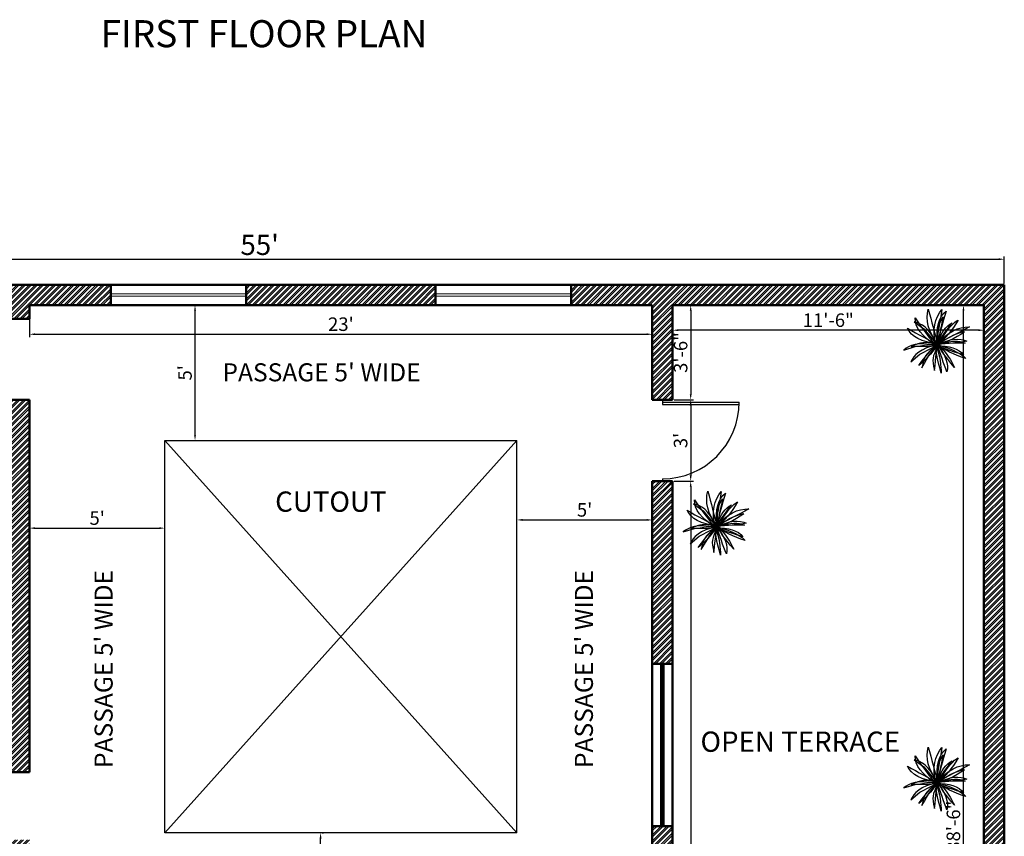
# Model space of a CAD drawing. Units: inches. Extents: x 3590 to 5167, y 65 to 1917.
# Tile 12 of 100: x 4644 to 5080, y 345 to 707. Entities that reach past the tile are written whole.
import ezdxf

# ---------------------------------------------------------------- set-up
doc = ezdxf.new("R2010")
doc.units = ezdxf.units.IN
for name, color, linetype, lineweight in [('A-ANNO-DIMS', 2, 'Continuous', 18), ('A-ANNO-TEXT', 7, 'Continuous', 25), ('A-AREA-IDEN', 7, 'Continuous', 18), ('A-DOOR', 3, 'Continuous', 25), ('A-FLOR-OTLN', 7, 'Continuous', 25), ('A-GLAZ', 4, 'Continuous', 18), ('A-WALL', 7, 'Continuous', 50), ('A-WALL-PATT', 251, 'Continuous', 13), ('L-PLNT', 94, 'Continuous', 18)]:
    doc.layers.add(name, color=color, linetype=linetype, lineweight=lineweight)
doc.layers.add('DIENHOA', color=3, linetype='Continuous')
doc.styles.get("Standard").update_dxf_attribs({"font": 'arial.ttf'})
doc.dimstyles.new('ISO-25', dxfattribs={"dimtxt": 9, "dimasz": 2.5, "dimexe": 1.25, "dimexo": 0.625, "dimtad": 1, "dimdec": 1, "dimlunit": 3, "dimtxsty": 'Standard', "dimcen": 2.5, "dimadec": 0, "dimazin": 0, "dimtfac": 1, "dimtdec": 1, "dimtmove": 0, "dimatfit": 3, "dimfxl": 1, "dimarcsym": 0})

# ---------------------------------------------------------------- blocks, each defined once
blk = doc.blocks.new('*D279')
at = {"layer": 'A-ANNO-DIMS', "color": 0, "lineweight": -2, "transparency": 16777216}
for p, q in [((4420.27, 589.68), (4420.27, 601.68)), ((4422.77, 600.43), (5077.77, 600.43)), ((5080.27, 589.68), (5080.27, 601.68))]:
    blk.add_line(p, q, dxfattribs=at)
at = {"layer": 'A-ANNO-DIMS', "color": 0, "transparency": 16777216}
for points in [[(4422.77, 600.84), (4422.77, 600.01), (4420.27, 600.43)], [(5077.77, 600.84), (5077.77, 600.01), (5080.27, 600.43)]]:
    blk.add_solid(points, dxfattribs=at)
at = {"layer": 'Defpoints', "color": 0, "transparency": 16777216}
for p in [(5080.27, 600.43), (4420.27, 589.06), (5080.27, 589.06)]:
    blk.add_point(p, dxfattribs=at)
at = {"layer": 'A-ANNO-DIMS', "color": 0, "transparency": 16777216, "insert": (4750.27, 605.63), "char_height": 9, "attachment_point": 5}
blk.add_mtext("55'", dxfattribs=at)
blk = doc.blocks.new('Cay03_mb')
at = {"layer": 'DIENHOA'}
for p, q in [((79, 504), (119, 555)), ((119, 555), (166, 599)), ((166, 599), (142, 519)), ((-365, 390), (-414, 403)), ((-414, 403), (-240, 278)), ((-315, 371), (-365, 390)), ((-264, 343), (-315, 371)), ((10, 295), (25, 374)), ((25, 374), (49, 444)), ((49, 444), (79, 504)), ((97, 366), (76, 291)), ((119, 442), (97, 366)), ((142, 519), (119, 442)), ((-211, 305), (-264, 343)), ((-240, 278), (-88, 95)), ((-158, 252), (-211, 305)), ((-104, 184), (-158, 252)), ((-50, 98), (-104, 184)), ((0, 105), (2, 206)), ((2, 206), (10, 295)), ((56, 216), (37, 142)), ((76, 291), (56, 216)), ((147, 144), (219, 200)), ((219, 200), (291, 243)), ((364, 193), (290, 155)), ((291, 243), (363, 275)), ((363, 275), (437, 297)), ((438, 231), (364, 193)), ((437, 297), (511, 310)), ((512, 271), (438, 231)), ((511, 310), (586, 314)), ((586, 314), (512, 271)), ((-345, 5), (-400, -17)), ((-299, 20), (-345, 5)), ((-255, 27), (-299, 20)), ((-208, 28), (-255, 27)), ((-153, 22), (-208, 28)), ((-83, 10), (-153, 22)), ((-88, 95), (5, -8)), ((5, -8), (-83, 10)), ((5, -8), (-50, 98)), ((5, -8), (0, 105)), ((5, -8), (76, 75)), ((20, 68), (5, -8)), ((75, 36), (5, -8)), ((5, -8), (100, 18)), ((46, 1), (5, -8)), ((37, 142), (20, 68)), ((97, 7), (46, 1)), ((145, 77), (75, 36)), ((76, 75), (147, 144)), ((155, 12), (97, 7)), ((100, 18), (182, 37)), ((217, 117), (145, 77)), ((220, 15), (155, 12)), ((182, 37), (253, 49)), ((290, 155), (217, 117)), ((289, 17), (220, 15)), ((253, 49), (315, 54)), ((362, 19), (289, 17)), ((315, 54), (369, 53)), ((436, 19), (362, 19)), ((369, 53), (419, 47)), ((419, 47), (465, 35)), ((510, 19), (436, 19)), ((465, 35), (510, 19)), ((-400, -17), (-468, -48)), ((-468, -48), (-376, -38)), ((-376, -38), (-295, -28)), ((-295, -28), (-226, -19)), ((-226, -19), (-166, -11)), ((-216, -236), (-166, -174)), ((-166, -11), (-114, -6)), ((-166, -174), (-120, -122)), ((-120, -122), (-80, -80)), ((-75, -127), (-118, -181)), ((-114, -6), (-69, -3)), ((-80, -80), (-45, -46)), ((-33, -69), (-75, -127)), ((-69, -3), (-30, -3)), ((-45, -46), (-17, -22)), ((5, -8), (-33, -69)), ((-30, -3), (5, -8)), ((-17, -22), (5, -8)), ((5, -8), (57, -73)), ((26, -64), (5, -8)), ((5, -8), (113, -40)), ((53, -42), (5, -8)), ((47, -126), (26, -64)), ((69, -191), (47, -126)), ((107, -76), (53, -42)), ((57, -73), (100, -139)), ((100, -139), (136, -204)), ((166, -110), (107, -76)), ((113, -40), (207, -74)), ((229, -143), (166, -110)), ((207, -74), (290, -108)), ((296, -175), (229, -143)), ((290, -108), (359, -141)), ((367, -205), (296, -175)), ((359, -141), (417, -174)), ((417, -174), (463, -204)), ((-330, -387), (-271, -307)), ((-291, -355), (-330, -387)), ((-250, -318), (-291, -355)), ((-271, -307), (-216, -236)), ((-206, -276), (-250, -318)), ((-162, -231), (-206, -276)), ((-118, -181), (-162, -231)), ((91, -257), (69, -191)), ((113, -322), (91, -257)), ((135, -386), (113, -322)), ((136, -204), (163, -268)), ((163, -268), (181, -330)), ((181, -330), (190, -390)), ((442, -233), (367, -205)), ((519, -258), (442, -233)), ((463, -204), (496, -232)), ((496, -232), (519, -258)), ((158, -445), (135, -386)), ((180, -499), (158, -445)), ((190, -446), (180, -499)), ((190, -390), (190, -446))]:
    blk.add_line(p, q, dxfattribs=at)
for points in [[(24, -5), (-41, 82), (-92, 167), (-130, 249), (-156, 330), (-170, 408), (-175, 484), (-170, 559), (-157, 633)], [(-157, 633), (-132, 551), (-111, 470), (-90, 389), (-70, 309), (-49, 229), (-27, 150), (-3, 72), (24, -5)], [(-16, -27), (-38, 80), (-49, 178), (-49, 269), (-39, 353), (-19, 430), (9, 501), (45, 567), (88, 629)], [(88, 629), (75, 544), (61, 461), (46, 379), (31, 298), (16, 217), (3, 136), (-8, 55), (-16, -27)], [(-396, 474), (-348, 406), (-301, 339), (-254, 275), (-208, 212), (-162, 151), (-115, 91), (-66, 32), (-16, -27)], [(-16, -27), (-108, 39), (-187, 102), (-252, 163), (-305, 224), (-345, 285), (-374, 347), (-390, 409), (-396, 474)], [(273, 387), (228, 329), (182, 270), (138, 212), (97, 156), (60, 103), (28, 55), (2, 11), (-16, -27)], [(-16, -27), (21, 64), (57, 140), (91, 203), (125, 255), (160, 297), (195, 332), (233, 362), (273, 387)], [(24, -5), (20, 93), (20, 177), (25, 249), (34, 310), (47, 363), (65, 409), (87, 452), (113, 492)], [(113, 492), (96, 420), (79, 347), (64, 276), (50, 208), (38, 145), (30, 87), (25, 36), (24, -5)], [(384, 437), (342, 368), (298, 302), (253, 239), (206, 181), (159, 127), (113, 78), (68, 34), (24, -5)], [(24, -5), (80, 92), (134, 176), (186, 248), (234, 309), (279, 357), (319, 395), (355, 421), (384, 437)], [(-530, 290), (-458, 248), (-388, 208), (-319, 169), (-251, 131), (-183, 95), (-115, 60), (-46, 26), (24, -5)], [(24, -5), (-87, 15), (-185, 40), (-270, 68), (-344, 101), (-406, 140), (-457, 184), (-499, 233), (-530, 290)], [(497, 224), (429, 178), (362, 137), (294, 99), (227, 66), (162, 37), (100, 11), (40, -10), (-16, -27)], [(-16, -27), (75, 38), (160, 92), (237, 136), (307, 170), (368, 195), (420, 213), (463, 222), (497, 224)], [(-16, -27), (-134, -5), (-235, 5), (-322, 5), (-396, -5), (-459, -22), (-512, -46), (-558, -74), (-598, -105)], [(24, -5), (99, 30), (173, 57), (245, 77), (313, 88), (378, 92), (438, 87), (493, 74), (541, 52)], [(541, 52), (484, 43), (421, 35), (354, 28), (285, 21), (216, 14), (148, 8), (83, 2), (24, -5)], [(-598, -105), (-393, -44), (-155, -37), (-16, -27)], [(-472, -320), (-310, -179), (-98, -73), (24, -5)], [(24, -5), (-92, -35), (-188, -68), (-267, -105), (-330, -145), (-380, -187), (-418, -231), (-448, -275), (-472, -320)], [(-276, -424), (-227, -345), (-186, -276), (-150, -216), (-119, -164), (-91, -120), (-66, -82), (-41, -52), (-16, -27)], [(-16, -27), (-85, -86), (-137, -133), (-176, -173), (-204, -210), (-226, -249), (-243, -295), (-258, -352), (-276, -424)], [(24, -5), (-14, -88), (-41, -153), (-60, -205), (-70, -251), (-73, -295), (-69, -344), (-60, -402), (-45, -475)], [(-45, -475), (-34, -383), (-25, -303), (-18, -233), (-12, -173), (-6, -121), (2, -77), (11, -39), (24, -5)], [(76, -524), (49, -428), (27, -342), (9, -264), (-4, -196), (-12, -138), (-17, -90), (-18, -53), (-16, -27)], [(478, -192), (422, -176), (361, -157), (298, -135), (232, -113), (167, -89), (102, -67), (41, -45), (-16, -27)], [(-16, -27), (67, -27), (146, -33), (219, -45), (286, -63), (346, -87), (398, -117), (443, -152), (478, -192)], [(-16, -27), (8, -95), (29, -163), (44, -231), (56, -296), (65, -359), (71, -419), (74, -474), (76, -524)], [(316, -418), (251, -343), (195, -273), (147, -210), (106, -154), (74, -105), (50, -63), (33, -30), (24, -5)], [(24, -5), (75, -57), (122, -111), (164, -165), (203, -219), (237, -273), (267, -324), (294, -373), (316, -418)]]:
    blk.add_lwpolyline(points, dxfattribs=at)
blk = doc.blocks.new('D1')
for p, q in [((1, 0), (1, 34)), ((2, 0), (2, 33.99)), ((0, 0), (2, 0)), ((35, 0), (36, 0))]:
    blk.add_line(p, q)
at = {"ltscale": 0.5}
blk.add_arc((1, 0), 34, 0, 90, dxfattribs=at)
blk = doc.blocks.new('*D256')
at = {"layer": 'A-ANNO-DIMS', "color": 0, "lineweight": -2, "transparency": 16777216}
for p, q in [((5070.65, 580.06), (5060.93, 580.06)), ((5062.18, 120.56), (5062.18, 577.56)), ((5070.65, 118.06), (5060.93, 118.06))]:
    blk.add_line(p, q, dxfattribs=at)
at = {"layer": 'A-ANNO-DIMS', "color": 0, "transparency": 16777216}
for points in [[(5061.77, 577.56), (5062.6, 577.56), (5062.18, 580.06)], [(5061.77, 120.56), (5062.6, 120.56), (5062.18, 118.06)]]:
    blk.add_solid(points, dxfattribs=at)
at = {"layer": 'Defpoints', "color": 0, "transparency": 16777216}
for p in [(5062.18, 580.06), (5071.27, 580.06), (5071.27, 118.06)]:
    blk.add_point(p, dxfattribs=at)
at = {"layer": 'A-ANNO-DIMS', "color": 0, "transparency": 16777216, "insert": (5058.49, 349.06), "char_height": 6, "attachment_point": 5, "rotation": 90}
blk.add_mtext('38\'-6"', dxfattribs=at)
blk = doc.blocks.new('*D233')
at = {"layer": 'A-ANNO-DIMS', "color": 0, "lineweight": -2, "transparency": 16777216}
for p, q in [((4933.27, 579.43), (4933.27, 567.69)), ((5071.27, 579.43), (5071.27, 567.69)), ((5068.77, 568.94), (4935.77, 568.94))]:
    blk.add_line(p, q, dxfattribs=at)
at = {"layer": 'A-ANNO-DIMS', "color": 0, "transparency": 16777216}
for points in [[(4935.77, 569.35), (4935.77, 568.52), (4933.27, 568.94)], [(5068.77, 569.35), (5068.77, 568.52), (5071.27, 568.94)]]:
    blk.add_solid(points, dxfattribs=at)
at = {"layer": 'Defpoints', "color": 0, "transparency": 16777216}
for p in [(4933.27, 580.06), (5071.27, 580.06), (4933.27, 568.94)]:
    blk.add_point(p, dxfattribs=at)
at = {"layer": 'A-ANNO-DIMS', "color": 0, "transparency": 16777216, "insert": (5002.27, 572.62), "char_height": 6, "attachment_point": 5}
blk.add_mtext('11\'-6"', dxfattribs=at)
blk = doc.blocks.new('*D234')
at = {"layer": 'A-ANNO-DIMS', "color": 0, "lineweight": -2, "transparency": 16777216}
for p, q in [((4933.9, 580.06), (4942.54, 580.06)), ((4941.29, 577.56), (4941.29, 540.56)), ((4933.9, 538.06), (4942.54, 538.06))]:
    blk.add_line(p, q, dxfattribs=at)
at = {"layer": 'A-ANNO-DIMS', "color": 0, "transparency": 16777216}
for points in [[(4940.87, 577.56), (4941.71, 577.56), (4941.29, 580.06)], [(4940.87, 540.56), (4941.71, 540.56), (4941.29, 538.06)]]:
    blk.add_solid(points, dxfattribs=at)
at = {"layer": 'Defpoints', "color": 0, "transparency": 16777216}
for p in [(4933.27, 580.06), (4933.27, 538.06), (4941.29, 538.06)]:
    blk.add_point(p, dxfattribs=at)
at = {"layer": 'A-ANNO-DIMS', "color": 0, "transparency": 16777216, "insert": (4937.6, 559.06), "char_height": 6, "attachment_point": 5, "rotation": 90}
blk.add_mtext('3\'-6"', dxfattribs=at)
blk = doc.blocks.new('*D235')
at = {"layer": 'A-ANNO-DIMS', "color": 0, "lineweight": -2, "transparency": 16777216}
for p, q in [((4933.9, 538.06), (4942.54, 538.06)), ((4941.29, 535.56), (4941.29, 504.56)), ((4933.9, 502.06), (4942.54, 502.06))]:
    blk.add_line(p, q, dxfattribs=at)
at = {"layer": 'A-ANNO-DIMS', "color": 0, "transparency": 16777216}
for points in [[(4940.87, 535.56), (4941.71, 535.56), (4941.29, 538.06)], [(4940.87, 504.56), (4941.71, 504.56), (4941.29, 502.06)]]:
    blk.add_solid(points, dxfattribs=at)
at = {"layer": 'Defpoints', "color": 0, "transparency": 16777216}
for p in [(4933.27, 538.06), (4933.27, 502.06), (4941.29, 502.06)]:
    blk.add_point(p, dxfattribs=at)
at = {"layer": 'A-ANNO-DIMS', "color": 0, "transparency": 16777216, "insert": (4937.6, 520.06), "char_height": 6, "attachment_point": 5, "rotation": 90}
blk.add_mtext("3'", dxfattribs=at)
blk = doc.blocks.new('*D236')
at = {"layer": 'A-ANNO-DIMS', "color": 0, "lineweight": -2, "transparency": 16777216}
for p, q in [((4933.9, 502.06), (4942.54, 502.06)), ((4941.29, 499.56), (4941.29, 120.56)), ((4933.9, 118.06), (4942.54, 118.06))]:
    blk.add_line(p, q, dxfattribs=at)
at = {"layer": 'A-ANNO-DIMS', "color": 0, "transparency": 16777216}
for points in [[(4940.87, 499.56), (4941.71, 499.56), (4941.29, 502.06)], [(4940.87, 120.56), (4941.71, 120.56), (4941.29, 118.06)]]:
    blk.add_solid(points, dxfattribs=at)
at = {"layer": 'Defpoints', "color": 0, "transparency": 16777216}
for p in [(4933.27, 502.06), (4933.27, 118.06), (4941.29, 118.06)]:
    blk.add_point(p, dxfattribs=at)
at = {"layer": 'A-ANNO-DIMS', "color": 0, "transparency": 16777216, "insert": (4937.6, 310.06), "char_height": 6, "attachment_point": 5, "rotation": 90}
blk.add_mtext("32'", dxfattribs=at)
blk = doc.blocks.new('*D237')
at = {"layer": 'A-ANNO-DIMS', "color": 0, "lineweight": -2, "transparency": 16777216}
for p, q in [((4648.27, 579.43), (4648.27, 565.9)), ((4924.27, 579.43), (4924.27, 565.9)), ((4650.77, 567.15), (4921.77, 567.15))]:
    blk.add_line(p, q, dxfattribs=at)
at = {"layer": 'A-ANNO-DIMS', "color": 0, "transparency": 16777216}
for points in [[(4650.77, 567.57), (4650.77, 566.74), (4648.27, 567.15)], [(4921.77, 567.57), (4921.77, 566.74), (4924.27, 567.15)]]:
    blk.add_solid(points, dxfattribs=at)
at = {"layer": 'Defpoints', "color": 0, "transparency": 16777216}
for p in [(4648.27, 580.06), (4924.27, 580.06), (4924.27, 567.15)]:
    blk.add_point(p, dxfattribs=at)
at = {"layer": 'A-ANNO-DIMS', "color": 0, "transparency": 16777216, "insert": (4786.27, 570.84), "char_height": 6, "attachment_point": 5}
blk.add_mtext("23'", dxfattribs=at)
blk = doc.blocks.new('*D229')
at = {"layer": 'A-ANNO-DIMS', "color": 0, "lineweight": -2, "transparency": 16777216}
for p, q in [((4648.27, 480.57), (4648.27, 479.94)), ((4650.77, 481.19), (4705.77, 481.19)), ((4708.27, 481.82), (4708.27, 482.44))]:
    blk.add_line(p, q, dxfattribs=at)
at = {"layer": 'A-ANNO-DIMS', "color": 0, "transparency": 16777216}
for points in [[(4650.77, 481.61), (4650.77, 480.78), (4648.27, 481.19)], [(4705.77, 481.61), (4705.77, 480.78), (4708.27, 481.19)]]:
    blk.add_solid(points, dxfattribs=at)
at = {"layer": 'Defpoints', "color": 0, "transparency": 16777216}
for p in [(4648.27, 481.19), (4708.27, 481.19), (4708.27, 481.19)]:
    blk.add_point(p, dxfattribs=at)
at = {"layer": 'A-ANNO-DIMS', "color": 0, "transparency": 16777216, "insert": (4678.27, 484.87), "char_height": 6, "attachment_point": 5}
blk.add_mtext("5'", dxfattribs=at)
blk = doc.blocks.new('*D230')
at = {"layer": 'A-ANNO-DIMS', "color": 0, "lineweight": -2, "transparency": 16777216}
for p, q in [((4721.63, 522.56), (4721.63, 577.56)), ((4722.25, 580.06), (4722.88, 580.06)), ((4722.25, 520.06), (4722.88, 520.06))]:
    blk.add_line(p, q, dxfattribs=at)
at = {"layer": 'A-ANNO-DIMS', "color": 0, "transparency": 16777216}
for points in [[(4721.21, 577.56), (4722.04, 577.56), (4721.63, 580.06)], [(4721.21, 522.56), (4722.04, 522.56), (4721.63, 520.06)]]:
    blk.add_solid(points, dxfattribs=at)
at = {"layer": 'Defpoints', "color": 0, "transparency": 16777216}
for p in [(4721.63, 580.06), (4721.63, 580.06), (4721.63, 520.06)]:
    blk.add_point(p, dxfattribs=at)
at = {"layer": 'A-ANNO-DIMS', "color": 0, "transparency": 16777216, "insert": (4717.95, 550.06), "char_height": 6, "attachment_point": 5, "rotation": 90}
blk.add_mtext("5'", dxfattribs=at)
blk = doc.blocks.new('*D231')
at = {"layer": 'A-ANNO-DIMS', "color": 0, "lineweight": -2, "transparency": 16777216}
for p, q in [((4777.9, 346.06), (4778.52, 346.06)), ((4777.27, 288.56), (4777.27, 343.56)), ((4777.9, 286.06), (4778.52, 286.06))]:
    blk.add_line(p, q, dxfattribs=at)
at = {"layer": 'A-ANNO-DIMS', "color": 0, "transparency": 16777216}
for points in [[(4776.86, 343.56), (4777.69, 343.56), (4777.27, 346.06)], [(4776.86, 288.56), (4777.69, 288.56), (4777.27, 286.06)]]:
    blk.add_solid(points, dxfattribs=at)
at = {"layer": 'Defpoints', "color": 0, "transparency": 16777216}
for p in [(4777.27, 346.06), (4777.27, 346.06), (4777.27, 286.06)]:
    blk.add_point(p, dxfattribs=at)
at = {"layer": 'A-ANNO-DIMS', "color": 0, "transparency": 16777216, "insert": (4773.6, 316.06), "char_height": 6, "attachment_point": 5, "rotation": 90}
blk.add_mtext("5'", dxfattribs=at)
blk = doc.blocks.new('*D232')
at = {"layer": 'A-ANNO-DIMS', "color": 0, "lineweight": -2, "transparency": 16777216}
for p, q in [((4864.27, 485.46), (4864.27, 486.08)), ((4866.77, 484.83), (4921.77, 484.83)), ((4924.27, 485.46), (4924.27, 486.08))]:
    blk.add_line(p, q, dxfattribs=at)
at = {"layer": 'A-ANNO-DIMS', "color": 0, "transparency": 16777216}
for points in [[(4866.77, 485.25), (4866.77, 484.42), (4864.27, 484.83)], [(4921.77, 485.25), (4921.77, 484.42), (4924.27, 484.83)]]:
    blk.add_solid(points, dxfattribs=at)
at = {"layer": 'Defpoints', "color": 0, "transparency": 16777216}
for p in [(4864.27, 484.83), (4924.27, 484.83), (4924.27, 484.83)]:
    blk.add_point(p, dxfattribs=at)
at = {"layer": 'A-ANNO-DIMS', "color": 0, "transparency": 16777216, "insert": (4894.27, 488.51), "char_height": 6, "attachment_point": 5}
blk.add_mtext("5'", dxfattribs=at)

msp = doc.modelspace()

# ---------------------------------------------------------------- hatches: boundary and pattern name
at = {"layer": 'A-WALL-PATT', "transparency": 33554687}
h = msp.add_hatch(dxfattribs=at)
h.set_pattern_fill('ANSI32', color=256, scale=0.2)
h.set_pattern_definition([(45, (0, -1216.9392), (-1.3470384, 1.3470384), []), (45, (0.898, -1216.9392), (-1.3470384, 1.3470384), [])])
h.paths.add_polyline_path([(4684.27, 589.06), (4591.27, 589.06), (4591.27, 580.06), (4639.27, 580.06), (4639.27, 574.06), (4648.27, 574.06), (4648.27, 580.06), (4684.27, 580.06)])
h.paths.add_polyline_path([(4543.27, 589.06), (4420.27, 589.06), (4420.27, 568.06), (4429.27, 568.06), (4429.27, 580.06), (4445.92, 580.06), (4543.27, 580.06)])
h.paths.add_polyline_path([(4828.27, 589.06), (4744.27, 589.06), (4744.27, 580.06), (4828.27, 580.06)])
h.paths.add_polyline_path([(4648.27, 538.06), (4639.27, 538.06), (4639.27, 439.06), (4546.27, 439.06), (4546.27, 433.06), (4549.27, 433.06), (4549.27, 337.06), (4429.27, 337.06), (4429.27, 367.06), (4420.27, 367.06), (4420.27, 322.06), (4429.27, 322.06), (4429.27, 328.06), (4639.27, 328.06), (4639.27, 322.06), (4648.27, 322.06), (4648.27, 343.06), (4639.27, 343.06), (4639.27, 337.06), (4555.27, 337.06), (4555.27, 433.06), (4639.27, 433.06), (4639.27, 373.06), (4648.27, 373.06)])
h.paths.add_polyline_path([(4516.27, 439.06), (4429.27, 439.06), (4429.27, 520.06), (4420.27, 520.06), (4420.27, 403.06), (4429.27, 403.06), (4429.27, 433.06), (4516.27, 433.06)], flags=17)
h.paths.add_polyline_path([(5080.27, 589.06), (4888.27, 589.06), (4888.27, 580.06), (4924.27, 580.06), (4924.27, 538.06), (4933.27, 538.06), (4933.27, 580.06), (5071.27, 580.06), (5071.27, 118.06), (4933.27, 118.06), (4933.27, 349.06), (4924.27, 349.06), (4924.27, 118.06), (4898.77, 118.06), (4898.77, 109.06), (5080.27, 109.06)])
h.paths.add_polyline_path([(4933.27, 502.06), (4924.27, 502.06), (4924.27, 421.06), (4933.27, 421.06)], flags=17)
h.paths.add_polyline_path([(4802.77, 118.06), (4777.27, 118.06), (4777.27, 286.06), (4756.27, 286.06), (4756.27, 277.06), (4768.27, 277.06), (4768.27, 214.06), (4696.27, 214.06), (4696.27, 277.06), (4708.27, 277.06), (4708.27, 286.06), (4639.27, 286.06), (4639.27, 277.06), (4687.27, 277.06), (4687.27, 214.06), (4681.27, 214.06), (4681.27, 205.06), (4768.27, 205.06), (4768.27, 118.06), (4726.27, 118.06), (4726.27, 109.06), (4802.77, 109.06)])
h.paths.add_polyline_path([(4690.27, 118.06), (4648.27, 118.06), (4648.27, 135.93), (4648.27, 205.06), (4651.27, 205.06), (4651.27, 214.06), (4639.27, 214.06), (4639.27, 118.06), (4633.27, 118.06), (4633.27, 109.06), (4690.27, 109.06)])
h.paths.add_polyline_path([(4585.27, 118.06), (4584.72, 118.06), (4429.27, 118.06), (4429.27, 274.06), (4420.27, 274.06), (4420.27, 109.06), (4585.27, 109.06)])

# ---------------------------------------------------------------- linework, layer by layer
at = {"layer": 'A-FLOR-OTLN'}
for p, q in [((4708.27, 520.06), (4864.27, 520.06)), ((4708.27, 346.06), (4708.27, 520.06)), ((4864.27, 346.06), (4864.27, 520.06)), ((4864.27, 346.06), (4708.27, 346.06))]:
    msp.add_line(p, q, dxfattribs=at)
at = {"layer": 'A-FLOR-OTLN', "ltscale": 0.5}
for p, q in [((4708.27, 520.06), (4864.27, 346.06)), ((4708.27, 346.06), (4864.27, 520.06))]:
    msp.add_line(p, q, dxfattribs=at)
at = {"layer": 'A-GLAZ'}
for p, q in [((4744.27, 585.06), (4684.27, 585.06)), ((4888.27, 585.06), (4828.27, 585.06)), ((4744.27, 584.06), (4684.27, 584.06)), ((4888.27, 584.06), (4828.27, 584.06))]:
    msp.add_line(p, q, dxfattribs=at)
at = {"layer": 'A-WALL'}
for p, q in [((4684.27, 580.06), (4684.27, 589.06)), ((4744.27, 580.06), (4744.27, 589.06)), ((4828.27, 580.06), (4828.27, 589.06)), ((4888.27, 580.06), (4888.27, 589.06)), ((4648.27, 580.06), (4924.27, 580.06)), ((4648.27, 574.06), (4648.27, 580.06)), ((4924.27, 538.06), (4924.27, 580.06)), ((4933.27, 580.06), (5071.27, 580.06)), ((4933.27, 538.06), (4933.27, 580.06)), ((5071.27, 118.06), (5071.27, 580.06)), ((4639.27, 574.06), (4648.27, 574.06)), ((4639.27, 538.06), (4648.27, 538.06)), ((4648.27, 373.06), (4648.27, 538.06)), ((4924.27, 538.06), (4933.27, 538.06)), ((4924.27, 118.06), (4924.27, 502.06)), ((4924.27, 502.06), (4933.27, 502.06)), ((4933.27, 118.06), (4933.27, 502.06)), ((4924.27, 421.06), (4933.27, 421.06)), ((4928.27, 349.06), (4928.27, 421.06)), ((4929.27, 349.06), (4929.27, 421.06)), ((4648.27, 373.06), (4639.27, 373.06)), ((4924.27, 349.06), (4933.27, 349.06))]:
    msp.add_line(p, q, dxfattribs=at)
msp.add_lwpolyline([(5080.27, 589.06), (5080.27, 109.06), (4420.27, 109.06), (4420.27, 589.06)], close=True, dxfattribs=at)

# ---------------------------------------------------------------- block references
at = {"layer": 'A-DOOR', "rotation": 270}
msp.add_blockref('D1', (4928.77, 538.06), dxfattribs=at)
at = {"layer": 'L-PLNT', "xscale": 0.0245452446402784, "yscale": 0.0245452446402784, "zscale": 0.0245452446402784}
for p in [(5050.43, 562.74), (4952.67, 482.06), (5050.43, 368.57)]:
    msp.add_blockref('Cay03_mb', p, dxfattribs=at)

# ---------------------------------------------------------------- texts
at = {"layer": 'A-ANNO-TEXT', "insert": (4679.79, 706.41), "char_height": 12, "attachment_point": 1}
msp.add_mtext_dynamic_manual_height_columns('{\\fTimes New Roman|b0|i0|c0|p18;FIRST FLOOR PLAN}', width=197.6934, gutter_width=12.5, heights=[0], dxfattribs=at)
at = {"layer": 'A-AREA-IDEN', "attachment_point": 1}
for s, width, insert, char_height in [("{\\fTimes New Roman|b0|i0|c0|p18;PASSAGE 5' WIDE}", 131.4857, (4733.77, 554.28), 8), ('{\\fTimes New Roman|b0|i0|c0|p18;CUTOUT}', 98.8219, (4757.14, 497.44), 9), ('{\\fTimes New Roman|b0|i0|c0|p18;OPEN TERRACE}', 98.8219, (4945.63, 391.02), 9)]:
    msp.add_mtext_dynamic_manual_height_columns(s, width=width, gutter_width=12.5, heights=[0], dxfattribs=dict(at, insert=insert, char_height=char_height))
at = {"layer": 'A-AREA-IDEN', "char_height": 8, "attachment_point": 1, "rotation": 90}
for insert in [(4677.11, 374.83), (4889.96, 374.83)]:
    msp.add_mtext_dynamic_manual_height_columns("{\\fTimes New Roman|b0|i0|c0|p18;PASSAGE 5' WIDE}", width=131.4857, gutter_width=12.5, heights=[0], dxfattribs=dict(at, insert=insert))

# ---------------------------------------------------------------- dimensions: what is measured, and where the dimension line sits
at = {"layer": 'A-ANNO-DIMS'}
for base, p1, p2, override, picture, middle in [((5080.27, 600.43), (4420.27, 589.06), (5080.27, 589.06), {"dimclrd": 0, "dimclre": 0, "dimclrt": 0}, '*D279', (4750.27, 605.63)), ((4924.27, 567.15), (4648.27, 580.06), (4924.27, 580.06), {"dimtxt": 6, "dimclrd": 0, "dimclre": 0, "dimclrt": 0}, '*D237', (4786.27, 570.84)), ((4933.27, 568.94), (5071.27, 580.06), (4933.27, 580.06), {"dimtxt": 6, "dimclrd": 0, "dimclre": 0, "dimclrt": 0}, '*D233', (5002.27, 572.62)), ((4708.27, 481.19), (4648.27, 481.19), (4708.27, 481.19), {"dimtxt": 6, "dimclrd": 0, "dimclre": 0, "dimclrt": 0}, '*D229', (4678.27, 484.87)), ((4924.27, 484.83), (4864.27, 484.83), (4924.27, 484.83), {"dimtxt": 6, "dimclrd": 0, "dimclre": 0, "dimclrt": 0}, '*D232', (4894.27, 488.51))]:
    dim = msp.add_linear_dim(base=base, p1=p1, p2=p2, dimstyle='ISO-25', override=override, dxfattribs=at)
    dim.commit()
    dim.dimension.update_dxf_attribs({"geometry": picture, "text_midpoint": middle})
for base, p1, p2, override, picture, middle in [((4721.63, 580.06), (4721.63, 520.06), (4721.63, 580.06), {"dimtxt": 6, "dimclrd": 0, "dimclre": 0, "dimclrt": 0}, '*D230', (4717.95, 550.06)), ((4941.29, 538.06), (4933.27, 580.06), (4933.27, 538.06), {"dimtxt": 6, "dimclrd": 0, "dimclre": 0, "dimclrt": 0}, '*D234', (4937.6, 559.06)), ((5062.18, 580.06), (5071.27, 118.06), (5071.27, 580.06), {"dimtxt": 6, "dimclrd": 0, "dimclre": 0, "dimclrt": 0}, '*D256', (5058.49, 349.06)), ((4941.29, 502.06), (4933.27, 538.06), (4933.27, 502.06), {"dimtxt": 6, "dimclrd": 0, "dimclre": 0, "dimclrt": 0, "dimtmove": 1}, '*D235', (4937.6, 520.06)), ((4941.29, 118.06), (4933.27, 502.06), (4933.27, 118.06), {"dimtxt": 6, "dimclrd": 0, "dimclre": 0, "dimclrt": 0, "dimtmove": 1}, '*D236', (4937.6, 310.06)), ((4777.27, 346.06), (4777.27, 286.06), (4777.27, 346.06), {"dimtxt": 6, "dimclrd": 0, "dimclre": 0, "dimclrt": 0}, '*D231', (4773.6, 316.06))]:
    dim = msp.add_linear_dim(base=base, p1=p1, p2=p2, angle=90, dimstyle='ISO-25', override=override, dxfattribs=at)
    dim.commit()
    dim.dimension.update_dxf_attribs({"geometry": picture, "text_midpoint": middle})

doc.saveas('drawing.dxf')
